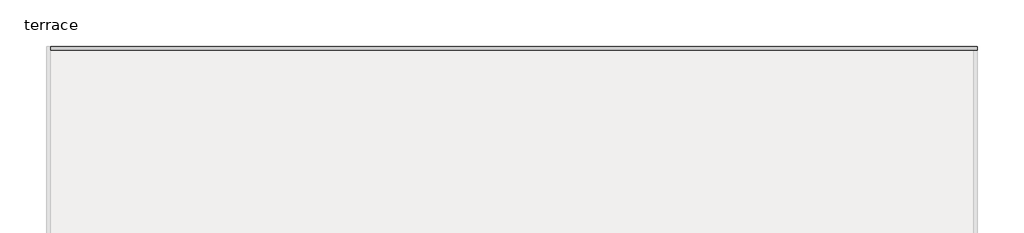
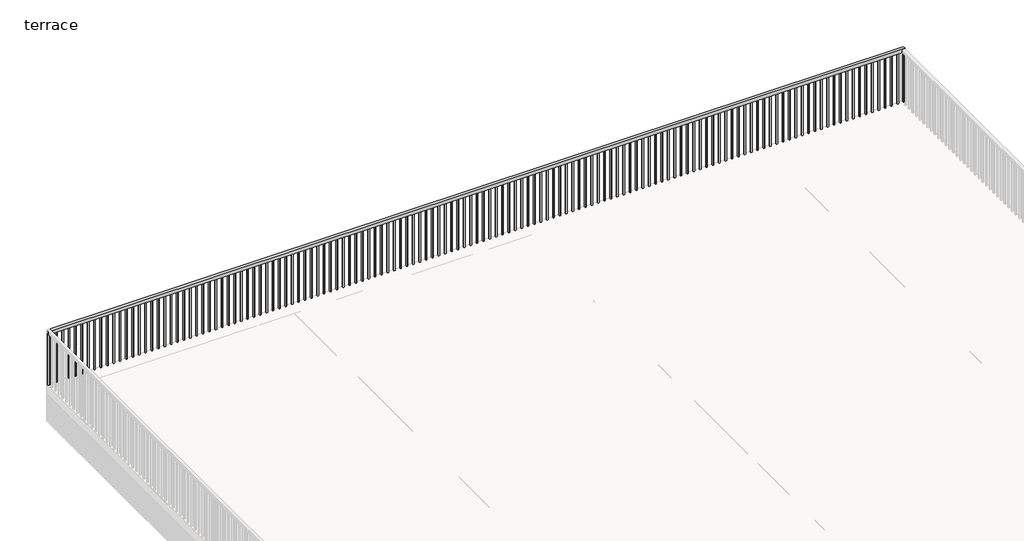
# One storey, part 5 of 6: 1 railing.
"""IFC4 building model written with IfcOpenShell, lengths in millimetres."""

from ifc_helpers import new_model, si_unit, frame, origin, place, context, project, spatial, polyline, outline, extrude, element, save

model = new_model("IFC4")

# Units and contexts
model_context = context("Model", 3, world=origin())
ifc_project = project(units=[si_unit("LENGTHUNIT", "METRE", prefix="MILLI")], contexts=[model_context])

# Site, building, storey
site = spatial("IfcSite", under=ifc_project)
building = spatial("IfcBuilding", under=site)
storey = spatial("IfcBuildingStorey", under=building, Name="terrace", Elevation=7010.4)

# Railing
placement = place(None, origin())
element("IfcRailing", 1, ObjectType="Handrail - Rectangular", at=placement, inside=storey, context=model_context, shape_type="SweptSolid", body=[
    extrude(outline(polyline([(-2647.3594779, 6526.2435985), (-2647.3594779, 6475.4435985), (-16300.5993763, 6475.4435985), (-16300.5993763, 6526.2435985), (-2647.3594779, 6526.2435985)])), frame((0.0, 0.0, 7874.0), z_axis=(0.0, 0.0, 1.0), x_axis=(1.0, 0.0, 0.0)), (0.0, 0.0, 1.0), 50.8),
    extrude(outline(polyline([(-16252.2344779, 6510.3685985), (-16252.2344779, 6491.3185985), (-16271.2844779, 6491.3185985), (-16271.2844779, 6510.3685985), (-16252.2344779, 6510.3685985)])), frame((0.0, 0.0, 7010.4), z_axis=(0.0, 0.0, 1.0), x_axis=(1.0, 0.0, 0.0)), (0.0, 0.0, 1.0), 863.6),
    extrude(outline(polyline([(-16150.6344779, 6510.3685985), (-16150.6344779, 6491.3185985), (-16169.6844779, 6491.3185985), (-16169.6844779, 6510.3685985), (-16150.6344779, 6510.3685985)])), frame((0.0, 0.0, 7010.4), z_axis=(0.0, 0.0, 1.0), x_axis=(1.0, 0.0, 0.0)), (0.0, 0.0, 1.0), 863.6),
    extrude(outline(polyline([(-16049.0344779, 6510.3685985), (-16049.0344779, 6491.3185985), (-16068.0844779, 6491.3185985), (-16068.0844779, 6510.3685985), (-16049.0344779, 6510.3685985)])), frame((0.0, 0.0, 7010.4), z_axis=(0.0, 0.0, 1.0), x_axis=(1.0, 0.0, 0.0)), (0.0, 0.0, 1.0), 863.6),
    extrude(outline(polyline([(-15947.4344779, 6510.3685985), (-15947.4344779, 6491.3185985), (-15966.4844779, 6491.3185985), (-15966.4844779, 6510.3685985), (-15947.4344779, 6510.3685985)])), frame((0.0, 0.0, 7010.4), z_axis=(0.0, 0.0, 1.0), x_axis=(1.0, 0.0, 0.0)), (0.0, 0.0, 1.0), 863.6),
    extrude(outline(polyline([(-15845.8344779, 6510.3685985), (-15845.8344779, 6491.3185985), (-15864.8844779, 6491.3185985), (-15864.8844779, 6510.3685985), (-15845.8344779, 6510.3685985)])), frame((0.0, 0.0, 7010.4), z_axis=(0.0, 0.0, 1.0), x_axis=(1.0, 0.0, 0.0)), (0.0, 0.0, 1.0), 863.6),
    extrude(outline(polyline([(-15744.2344779, 6510.3685985), (-15744.2344779, 6491.3185985), (-15763.2844779, 6491.3185985), (-15763.2844779, 6510.3685985), (-15744.2344779, 6510.3685985)])), frame((0.0, 0.0, 7010.4), z_axis=(0.0, 0.0, 1.0), x_axis=(1.0, 0.0, 0.0)), (0.0, 0.0, 1.0), 863.6),
    extrude(outline(polyline([(-15642.6344779, 6510.3685985), (-15642.6344779, 6491.3185985), (-15661.6844779, 6491.3185985), (-15661.6844779, 6510.3685985), (-15642.6344779, 6510.3685985)])), frame((0.0, 0.0, 7010.4), z_axis=(0.0, 0.0, 1.0), x_axis=(1.0, 0.0, 0.0)), (0.0, 0.0, 1.0), 863.6),
    extrude(outline(polyline([(-15541.0344779, 6510.3685985), (-15541.0344779, 6491.3185985), (-15560.0844779, 6491.3185985), (-15560.0844779, 6510.3685985), (-15541.0344779, 6510.3685985)])), frame((0.0, 0.0, 7010.4), z_axis=(0.0, 0.0, 1.0), x_axis=(1.0, 0.0, 0.0)), (0.0, 0.0, 1.0), 863.6),
    extrude(outline(polyline([(-15439.4344779, 6510.3685985), (-15439.4344779, 6491.3185985), (-15458.4844779, 6491.3185985), (-15458.4844779, 6510.3685985), (-15439.4344779, 6510.3685985)])), frame((0.0, 0.0, 7010.4), z_axis=(0.0, 0.0, 1.0), x_axis=(1.0, 0.0, 0.0)), (0.0, 0.0, 1.0), 863.6),
    extrude(outline(polyline([(-15337.8344779, 6510.3685985), (-15337.8344779, 6491.3185985), (-15356.8844779, 6491.3185985), (-15356.8844779, 6510.3685985), (-15337.8344779, 6510.3685985)])), frame((0.0, 0.0, 7010.4), z_axis=(0.0, 0.0, 1.0), x_axis=(1.0, 0.0, 0.0)), (0.0, 0.0, 1.0), 863.6),
    extrude(outline(polyline([(-15236.2344779, 6510.3685985), (-15236.2344779, 6491.3185985), (-15255.2844779, 6491.3185985), (-15255.2844779, 6510.3685985), (-15236.2344779, 6510.3685985)])), frame((0.0, 0.0, 7010.4), z_axis=(0.0, 0.0, 1.0), x_axis=(1.0, 0.0, 0.0)), (0.0, 0.0, 1.0), 863.6),
    extrude(outline(polyline([(-15134.6344779, 6510.3685985), (-15134.6344779, 6491.3185985), (-15153.6844779, 6491.3185985), (-15153.6844779, 6510.3685985), (-15134.6344779, 6510.3685985)])), frame((0.0, 0.0, 7010.4), z_axis=(0.0, 0.0, 1.0), x_axis=(1.0, 0.0, 0.0)), (0.0, 0.0, 1.0), 863.6),
    extrude(outline(polyline([(-15033.0344779, 6510.3685985), (-15033.0344779, 6491.3185985), (-15052.0844779, 6491.3185985), (-15052.0844779, 6510.3685985), (-15033.0344779, 6510.3685985)])), frame((0.0, 0.0, 7010.4), z_axis=(0.0, 0.0, 1.0), x_axis=(1.0, 0.0, 0.0)), (0.0, 0.0, 1.0), 863.6),
    extrude(outline(polyline([(-14931.4344779, 6510.3685985), (-14931.4344779, 6491.3185985), (-14950.4844779, 6491.3185985), (-14950.4844779, 6510.3685985), (-14931.4344779, 6510.3685985)])), frame((0.0, 0.0, 7010.4), z_axis=(0.0, 0.0, 1.0), x_axis=(1.0, 0.0, 0.0)), (0.0, 0.0, 1.0), 863.6),
    extrude(outline(polyline([(-14829.8344779, 6510.3685985), (-14829.8344779, 6491.3185985), (-14848.8844779, 6491.3185985), (-14848.8844779, 6510.3685985), (-14829.8344779, 6510.3685985)])), frame((0.0, 0.0, 7010.4), z_axis=(0.0, 0.0, 1.0), x_axis=(1.0, 0.0, 0.0)), (0.0, 0.0, 1.0), 863.6),
    extrude(outline(polyline([(-14728.2344779, 6510.3685985), (-14728.2344779, 6491.3185985), (-14747.2844779, 6491.3185985), (-14747.2844779, 6510.3685985), (-14728.2344779, 6510.3685985)])), frame((0.0, 0.0, 7010.4), z_axis=(0.0, 0.0, 1.0), x_axis=(1.0, 0.0, 0.0)), (0.0, 0.0, 1.0), 863.6),
    extrude(outline(polyline([(-14626.6344779, 6510.3685985), (-14626.6344779, 6491.3185985), (-14645.6844779, 6491.3185985), (-14645.6844779, 6510.3685985), (-14626.6344779, 6510.3685985)])), frame((0.0, 0.0, 7010.4), z_axis=(0.0, 0.0, 1.0), x_axis=(1.0, 0.0, 0.0)), (0.0, 0.0, 1.0), 863.6),
    extrude(outline(polyline([(-14525.0344779, 6510.3685985), (-14525.0344779, 6491.3185985), (-14544.0844779, 6491.3185985), (-14544.0844779, 6510.3685985), (-14525.0344779, 6510.3685985)])), frame((0.0, 0.0, 7010.4), z_axis=(0.0, 0.0, 1.0), x_axis=(1.0, 0.0, 0.0)), (0.0, 0.0, 1.0), 863.6),
    extrude(outline(polyline([(-14423.4344779, 6510.3685985), (-14423.4344779, 6491.3185985), (-14442.4844779, 6491.3185985), (-14442.4844779, 6510.3685985), (-14423.4344779, 6510.3685985)])), frame((0.0, 0.0, 7010.4), z_axis=(0.0, 0.0, 1.0), x_axis=(1.0, 0.0, 0.0)), (0.0, 0.0, 1.0), 863.6),
    extrude(outline(polyline([(-14321.8344779, 6510.3685985), (-14321.8344779, 6491.3185985), (-14340.8844779, 6491.3185985), (-14340.8844779, 6510.3685985), (-14321.8344779, 6510.3685985)])), frame((0.0, 0.0, 7010.4), z_axis=(0.0, 0.0, 1.0), x_axis=(1.0, 0.0, 0.0)), (0.0, 0.0, 1.0), 863.6),
    extrude(outline(polyline([(-14220.2344779, 6510.3685985), (-14220.2344779, 6491.3185985), (-14239.2844779, 6491.3185985), (-14239.2844779, 6510.3685985), (-14220.2344779, 6510.3685985)])), frame((0.0, 0.0, 7010.4), z_axis=(0.0, 0.0, 1.0), x_axis=(1.0, 0.0, 0.0)), (0.0, 0.0, 1.0), 863.6),
    extrude(outline(polyline([(-14118.6344779, 6510.3685985), (-14118.6344779, 6491.3185985), (-14137.6844779, 6491.3185985), (-14137.6844779, 6510.3685985), (-14118.6344779, 6510.3685985)])), frame((0.0, 0.0, 7010.4), z_axis=(0.0, 0.0, 1.0), x_axis=(1.0, 0.0, 0.0)), (0.0, 0.0, 1.0), 863.6),
    extrude(outline(polyline([(-14017.0344779, 6510.3685985), (-14017.0344779, 6491.3185985), (-14036.0844779, 6491.3185985), (-14036.0844779, 6510.3685985), (-14017.0344779, 6510.3685985)])), frame((0.0, 0.0, 7010.4), z_axis=(0.0, 0.0, 1.0), x_axis=(1.0, 0.0, 0.0)), (0.0, 0.0, 1.0), 863.6),
    extrude(outline(polyline([(-13915.4344779, 6510.3685985), (-13915.4344779, 6491.3185985), (-13934.4844779, 6491.3185985), (-13934.4844779, 6510.3685985), (-13915.4344779, 6510.3685985)])), frame((0.0, 0.0, 7010.4), z_axis=(0.0, 0.0, 1.0), x_axis=(1.0, 0.0, 0.0)), (0.0, 0.0, 1.0), 863.6),
    extrude(outline(polyline([(-13813.8344779, 6510.3685985), (-13813.8344779, 6491.3185985), (-13832.8844779, 6491.3185985), (-13832.8844779, 6510.3685985), (-13813.8344779, 6510.3685985)])), frame((0.0, 0.0, 7010.4), z_axis=(0.0, 0.0, 1.0), x_axis=(1.0, 0.0, 0.0)), (0.0, 0.0, 1.0), 863.6),
    extrude(outline(polyline([(-13712.2344779, 6510.3685985), (-13712.2344779, 6491.3185985), (-13731.2844779, 6491.3185985), (-13731.2844779, 6510.3685985), (-13712.2344779, 6510.3685985)])), frame((0.0, 0.0, 7010.4), z_axis=(0.0, 0.0, 1.0), x_axis=(1.0, 0.0, 0.0)), (0.0, 0.0, 1.0), 863.6),
    extrude(outline(polyline([(-13610.6344779, 6510.3685985), (-13610.6344779, 6491.3185985), (-13629.6844779, 6491.3185985), (-13629.6844779, 6510.3685985), (-13610.6344779, 6510.3685985)])), frame((0.0, 0.0, 7010.4), z_axis=(0.0, 0.0, 1.0), x_axis=(1.0, 0.0, 0.0)), (0.0, 0.0, 1.0), 863.6),
    extrude(outline(polyline([(-13509.0344779, 6510.3685985), (-13509.0344779, 6491.3185985), (-13528.0844779, 6491.3185985), (-13528.0844779, 6510.3685985), (-13509.0344779, 6510.3685985)])), frame((0.0, 0.0, 7010.4), z_axis=(0.0, 0.0, 1.0), x_axis=(1.0, 0.0, 0.0)), (0.0, 0.0, 1.0), 863.6),
    extrude(outline(polyline([(-13407.4344779, 6510.3685985), (-13407.4344779, 6491.3185985), (-13426.4844779, 6491.3185985), (-13426.4844779, 6510.3685985), (-13407.4344779, 6510.3685985)])), frame((0.0, 0.0, 7010.4), z_axis=(0.0, 0.0, 1.0), x_axis=(1.0, 0.0, 0.0)), (0.0, 0.0, 1.0), 863.6),
    extrude(outline(polyline([(-13305.8344779, 6510.3685985), (-13305.8344779, 6491.3185985), (-13324.8844779, 6491.3185985), (-13324.8844779, 6510.3685985), (-13305.8344779, 6510.3685985)])), frame((0.0, 0.0, 7010.4), z_axis=(0.0, 0.0, 1.0), x_axis=(1.0, 0.0, 0.0)), (0.0, 0.0, 1.0), 863.6),
    extrude(outline(polyline([(-13204.2344779, 6510.3685985), (-13204.2344779, 6491.3185985), (-13223.2844779, 6491.3185985), (-13223.2844779, 6510.3685985), (-13204.2344779, 6510.3685985)])), frame((0.0, 0.0, 7010.4), z_axis=(0.0, 0.0, 1.0), x_axis=(1.0, 0.0, 0.0)), (0.0, 0.0, 1.0), 863.6),
    extrude(outline(polyline([(-13102.6344779, 6510.3685985), (-13102.6344779, 6491.3185985), (-13121.6844779, 6491.3185985), (-13121.6844779, 6510.3685985), (-13102.6344779, 6510.3685985)])), frame((0.0, 0.0, 7010.4), z_axis=(0.0, 0.0, 1.0), x_axis=(1.0, 0.0, 0.0)), (0.0, 0.0, 1.0), 863.6),
    extrude(outline(polyline([(-13001.0344779, 6510.3685985), (-13001.0344779, 6491.3185985), (-13020.0844779, 6491.3185985), (-13020.0844779, 6510.3685985), (-13001.0344779, 6510.3685985)])), frame((0.0, 0.0, 7010.4), z_axis=(0.0, 0.0, 1.0), x_axis=(1.0, 0.0, 0.0)), (0.0, 0.0, 1.0), 863.6),
    extrude(outline(polyline([(-12899.4344779, 6510.3685985), (-12899.4344779, 6491.3185985), (-12918.4844779, 6491.3185985), (-12918.4844779, 6510.3685985), (-12899.4344779, 6510.3685985)])), frame((0.0, 0.0, 7010.4), z_axis=(0.0, 0.0, 1.0), x_axis=(1.0, 0.0, 0.0)), (0.0, 0.0, 1.0), 863.6),
    extrude(outline(polyline([(-12797.8344779, 6510.3685985), (-12797.8344779, 6491.3185985), (-12816.8844779, 6491.3185985), (-12816.8844779, 6510.3685985), (-12797.8344779, 6510.3685985)])), frame((0.0, 0.0, 7010.4), z_axis=(0.0, 0.0, 1.0), x_axis=(1.0, 0.0, 0.0)), (0.0, 0.0, 1.0), 863.6),
    extrude(outline(polyline([(-12696.2344779, 6510.3685985), (-12696.2344779, 6491.3185985), (-12715.2844779, 6491.3185985), (-12715.2844779, 6510.3685985), (-12696.2344779, 6510.3685985)])), frame((0.0, 0.0, 7010.4), z_axis=(0.0, 0.0, 1.0), x_axis=(1.0, 0.0, 0.0)), (0.0, 0.0, 1.0), 863.6),
    extrude(outline(polyline([(-12594.6344779, 6510.3685985), (-12594.6344779, 6491.3185985), (-12613.6844779, 6491.3185985), (-12613.6844779, 6510.3685985), (-12594.6344779, 6510.3685985)])), frame((0.0, 0.0, 7010.4), z_axis=(0.0, 0.0, 1.0), x_axis=(1.0, 0.0, 0.0)), (0.0, 0.0, 1.0), 863.6),
    extrude(outline(polyline([(-12493.0344779, 6510.3685985), (-12493.0344779, 6491.3185985), (-12512.0844779, 6491.3185985), (-12512.0844779, 6510.3685985), (-12493.0344779, 6510.3685985)])), frame((0.0, 0.0, 7010.4), z_axis=(0.0, 0.0, 1.0), x_axis=(1.0, 0.0, 0.0)), (0.0, 0.0, 1.0), 863.6),
    extrude(outline(polyline([(-12391.4344779, 6510.3685985), (-12391.4344779, 6491.3185985), (-12410.4844779, 6491.3185985), (-12410.4844779, 6510.3685985), (-12391.4344779, 6510.3685985)])), frame((0.0, 0.0, 7010.4), z_axis=(0.0, 0.0, 1.0), x_axis=(1.0, 0.0, 0.0)), (0.0, 0.0, 1.0), 863.6),
    extrude(outline(polyline([(-12289.8344779, 6510.3685985), (-12289.8344779, 6491.3185985), (-12308.8844779, 6491.3185985), (-12308.8844779, 6510.3685985), (-12289.8344779, 6510.3685985)])), frame((0.0, 0.0, 7010.4), z_axis=(0.0, 0.0, 1.0), x_axis=(1.0, 0.0, 0.0)), (0.0, 0.0, 1.0), 863.6),
    extrude(outline(polyline([(-12188.2344779, 6510.3685985), (-12188.2344779, 6491.3185985), (-12207.2844779, 6491.3185985), (-12207.2844779, 6510.3685985), (-12188.2344779, 6510.3685985)])), frame((0.0, 0.0, 7010.4), z_axis=(0.0, 0.0, 1.0), x_axis=(1.0, 0.0, 0.0)), (0.0, 0.0, 1.0), 863.6),
    extrude(outline(polyline([(-12086.6344779, 6510.3685985), (-12086.6344779, 6491.3185985), (-12105.6844779, 6491.3185985), (-12105.6844779, 6510.3685985), (-12086.6344779, 6510.3685985)])), frame((0.0, 0.0, 7010.4), z_axis=(0.0, 0.0, 1.0), x_axis=(1.0, 0.0, 0.0)), (0.0, 0.0, 1.0), 863.6),
    extrude(outline(polyline([(-11985.0344779, 6510.3685985), (-11985.0344779, 6491.3185985), (-12004.0844779, 6491.3185985), (-12004.0844779, 6510.3685985), (-11985.0344779, 6510.3685985)])), frame((0.0, 0.0, 7010.4), z_axis=(0.0, 0.0, 1.0), x_axis=(1.0, 0.0, 0.0)), (0.0, 0.0, 1.0), 863.6),
    extrude(outline(polyline([(-11883.4344779, 6510.3685985), (-11883.4344779, 6491.3185985), (-11902.4844779, 6491.3185985), (-11902.4844779, 6510.3685985), (-11883.4344779, 6510.3685985)])), frame((0.0, 0.0, 7010.4), z_axis=(0.0, 0.0, 1.0), x_axis=(1.0, 0.0, 0.0)), (0.0, 0.0, 1.0), 863.6),
    extrude(outline(polyline([(-11781.8344779, 6510.3685985), (-11781.8344779, 6491.3185985), (-11800.8844779, 6491.3185985), (-11800.8844779, 6510.3685985), (-11781.8344779, 6510.3685985)])), frame((0.0, 0.0, 7010.4), z_axis=(0.0, 0.0, 1.0), x_axis=(1.0, 0.0, 0.0)), (0.0, 0.0, 1.0), 863.6),
    extrude(outline(polyline([(-11680.2344779, 6510.3685985), (-11680.2344779, 6491.3185985), (-11699.2844779, 6491.3185985), (-11699.2844779, 6510.3685985), (-11680.2344779, 6510.3685985)])), frame((0.0, 0.0, 7010.4), z_axis=(0.0, 0.0, 1.0), x_axis=(1.0, 0.0, 0.0)), (0.0, 0.0, 1.0), 863.6),
    extrude(outline(polyline([(-11578.6344779, 6510.3685985), (-11578.6344779, 6491.3185985), (-11597.6844779, 6491.3185985), (-11597.6844779, 6510.3685985), (-11578.6344779, 6510.3685985)])), frame((0.0, 0.0, 7010.4), z_axis=(0.0, 0.0, 1.0), x_axis=(1.0, 0.0, 0.0)), (0.0, 0.0, 1.0), 863.6),
    extrude(outline(polyline([(-11477.0344779, 6510.3685985), (-11477.0344779, 6491.3185985), (-11496.0844779, 6491.3185985), (-11496.0844779, 6510.3685985), (-11477.0344779, 6510.3685985)])), frame((0.0, 0.0, 7010.4), z_axis=(0.0, 0.0, 1.0), x_axis=(1.0, 0.0, 0.0)), (0.0, 0.0, 1.0), 863.6),
    extrude(outline(polyline([(-11375.4344779, 6510.3685985), (-11375.4344779, 6491.3185985), (-11394.4844779, 6491.3185985), (-11394.4844779, 6510.3685985), (-11375.4344779, 6510.3685985)])), frame((0.0, 0.0, 7010.4), z_axis=(0.0, 0.0, 1.0), x_axis=(1.0, 0.0, 0.0)), (0.0, 0.0, 1.0), 863.6),
    extrude(outline(polyline([(-11273.8344779, 6510.3685985), (-11273.8344779, 6491.3185985), (-11292.8844779, 6491.3185985), (-11292.8844779, 6510.3685985), (-11273.8344779, 6510.3685985)])), frame((0.0, 0.0, 7010.4), z_axis=(0.0, 0.0, 1.0), x_axis=(1.0, 0.0, 0.0)), (0.0, 0.0, 1.0), 863.6),
    extrude(outline(polyline([(-11172.2344779, 6510.3685985), (-11172.2344779, 6491.3185985), (-11191.2844779, 6491.3185985), (-11191.2844779, 6510.3685985), (-11172.2344779, 6510.3685985)])), frame((0.0, 0.0, 7010.4), z_axis=(0.0, 0.0, 1.0), x_axis=(1.0, 0.0, 0.0)), (0.0, 0.0, 1.0), 863.6),
    extrude(outline(polyline([(-11070.6344779, 6510.3685985), (-11070.6344779, 6491.3185985), (-11089.6844779, 6491.3185985), (-11089.6844779, 6510.3685985), (-11070.6344779, 6510.3685985)])), frame((0.0, 0.0, 7010.4), z_axis=(0.0, 0.0, 1.0), x_axis=(1.0, 0.0, 0.0)), (0.0, 0.0, 1.0), 863.6),
    extrude(outline(polyline([(-10969.0344779, 6510.3685985), (-10969.0344779, 6491.3185985), (-10988.0844779, 6491.3185985), (-10988.0844779, 6510.3685985), (-10969.0344779, 6510.3685985)])), frame((0.0, 0.0, 7010.4), z_axis=(0.0, 0.0, 1.0), x_axis=(1.0, 0.0, 0.0)), (0.0, 0.0, 1.0), 863.6),
    extrude(outline(polyline([(-10867.4344779, 6510.3685985), (-10867.4344779, 6491.3185985), (-10886.4844779, 6491.3185985), (-10886.4844779, 6510.3685985), (-10867.4344779, 6510.3685985)])), frame((0.0, 0.0, 7010.4), z_axis=(0.0, 0.0, 1.0), x_axis=(1.0, 0.0, 0.0)), (0.0, 0.0, 1.0), 863.6),
    extrude(outline(polyline([(-10765.8344779, 6510.3685985), (-10765.8344779, 6491.3185985), (-10784.8844779, 6491.3185985), (-10784.8844779, 6510.3685985), (-10765.8344779, 6510.3685985)])), frame((0.0, 0.0, 7010.4), z_axis=(0.0, 0.0, 1.0), x_axis=(1.0, 0.0, 0.0)), (0.0, 0.0, 1.0), 863.6),
    extrude(outline(polyline([(-10664.2344779, 6510.3685985), (-10664.2344779, 6491.3185985), (-10683.2844779, 6491.3185985), (-10683.2844779, 6510.3685985), (-10664.2344779, 6510.3685985)])), frame((0.0, 0.0, 7010.4), z_axis=(0.0, 0.0, 1.0), x_axis=(1.0, 0.0, 0.0)), (0.0, 0.0, 1.0), 863.6),
    extrude(outline(polyline([(-10562.6344779, 6510.3685985), (-10562.6344779, 6491.3185985), (-10581.6844779, 6491.3185985), (-10581.6844779, 6510.3685985), (-10562.6344779, 6510.3685985)])), frame((0.0, 0.0, 7010.4), z_axis=(0.0, 0.0, 1.0), x_axis=(1.0, 0.0, 0.0)), (0.0, 0.0, 1.0), 863.6),
    extrude(outline(polyline([(-10461.0344779, 6510.3685985), (-10461.0344779, 6491.3185985), (-10480.0844779, 6491.3185985), (-10480.0844779, 6510.3685985), (-10461.0344779, 6510.3685985)])), frame((0.0, 0.0, 7010.4), z_axis=(0.0, 0.0, 1.0), x_axis=(1.0, 0.0, 0.0)), (0.0, 0.0, 1.0), 863.6),
    extrude(outline(polyline([(-10359.4344779, 6510.3685985), (-10359.4344779, 6491.3185985), (-10378.4844779, 6491.3185985), (-10378.4844779, 6510.3685985), (-10359.4344779, 6510.3685985)])), frame((0.0, 0.0, 7010.4), z_axis=(0.0, 0.0, 1.0), x_axis=(1.0, 0.0, 0.0)), (0.0, 0.0, 1.0), 863.6),
    extrude(outline(polyline([(-10257.8344779, 6510.3685985), (-10257.8344779, 6491.3185985), (-10276.8844779, 6491.3185985), (-10276.8844779, 6510.3685985), (-10257.8344779, 6510.3685985)])), frame((0.0, 0.0, 7010.4), z_axis=(0.0, 0.0, 1.0), x_axis=(1.0, 0.0, 0.0)), (0.0, 0.0, 1.0), 863.6),
    extrude(outline(polyline([(-10156.2344779, 6510.3685985), (-10156.2344779, 6491.3185985), (-10175.2844779, 6491.3185985), (-10175.2844779, 6510.3685985), (-10156.2344779, 6510.3685985)])), frame((0.0, 0.0, 7010.4), z_axis=(0.0, 0.0, 1.0), x_axis=(1.0, 0.0, 0.0)), (0.0, 0.0, 1.0), 863.6),
    extrude(outline(polyline([(-10054.6344779, 6510.3685985), (-10054.6344779, 6491.3185985), (-10073.6844779, 6491.3185985), (-10073.6844779, 6510.3685985), (-10054.6344779, 6510.3685985)])), frame((0.0, 0.0, 7010.4), z_axis=(0.0, 0.0, 1.0), x_axis=(1.0, 0.0, 0.0)), (0.0, 0.0, 1.0), 863.6),
    extrude(outline(polyline([(-9953.0344779, 6510.3685985), (-9953.0344779, 6491.3185985), (-9972.0844779, 6491.3185985), (-9972.0844779, 6510.3685985), (-9953.0344779, 6510.3685985)])), frame((0.0, 0.0, 7010.4), z_axis=(0.0, 0.0, 1.0), x_axis=(1.0, 0.0, 0.0)), (0.0, 0.0, 1.0), 863.6),
    extrude(outline(polyline([(-9851.4344779, 6510.3685985), (-9851.4344779, 6491.3185985), (-9870.4844779, 6491.3185985), (-9870.4844779, 6510.3685985), (-9851.4344779, 6510.3685985)])), frame((0.0, 0.0, 7010.4), z_axis=(0.0, 0.0, 1.0), x_axis=(1.0, 0.0, 0.0)), (0.0, 0.0, 1.0), 863.6),
    extrude(outline(polyline([(-9749.8344779, 6510.3685985), (-9749.8344779, 6491.3185985), (-9768.8844779, 6491.3185985), (-9768.8844779, 6510.3685985), (-9749.8344779, 6510.3685985)])), frame((0.0, 0.0, 7010.4), z_axis=(0.0, 0.0, 1.0), x_axis=(1.0, 0.0, 0.0)), (0.0, 0.0, 1.0), 863.6),
    extrude(outline(polyline([(-9648.2344779, 6510.3685985), (-9648.2344779, 6491.3185985), (-9667.2844779, 6491.3185985), (-9667.2844779, 6510.3685985), (-9648.2344779, 6510.3685985)])), frame((0.0, 0.0, 7010.4), z_axis=(0.0, 0.0, 1.0), x_axis=(1.0, 0.0, 0.0)), (0.0, 0.0, 1.0), 863.6),
    extrude(outline(polyline([(-9546.6344779, 6510.3685985), (-9546.6344779, 6491.3185985), (-9565.6844779, 6491.3185985), (-9565.6844779, 6510.3685985), (-9546.6344779, 6510.3685985)])), frame((0.0, 0.0, 7010.4), z_axis=(0.0, 0.0, 1.0), x_axis=(1.0, 0.0, 0.0)), (0.0, 0.0, 1.0), 863.6),
    extrude(outline(polyline([(-9445.0344779, 6510.3685985), (-9445.0344779, 6491.3185985), (-9464.0844779, 6491.3185985), (-9464.0844779, 6510.3685985), (-9445.0344779, 6510.3685985)])), frame((0.0, 0.0, 7010.4), z_axis=(0.0, 0.0, 1.0), x_axis=(1.0, 0.0, 0.0)), (0.0, 0.0, 1.0), 863.6),
    extrude(outline(polyline([(-9343.4344779, 6510.3685985), (-9343.4344779, 6491.3185985), (-9362.4844779, 6491.3185985), (-9362.4844779, 6510.3685985), (-9343.4344779, 6510.3685985)])), frame((0.0, 0.0, 7010.4), z_axis=(0.0, 0.0, 1.0), x_axis=(1.0, 0.0, 0.0)), (0.0, 0.0, 1.0), 863.6),
    extrude(outline(polyline([(-9241.8344779, 6510.3685985), (-9241.8344779, 6491.3185985), (-9260.8844779, 6491.3185985), (-9260.8844779, 6510.3685985), (-9241.8344779, 6510.3685985)])), frame((0.0, 0.0, 7010.4), z_axis=(0.0, 0.0, 1.0), x_axis=(1.0, 0.0, 0.0)), (0.0, 0.0, 1.0), 863.6),
    extrude(outline(polyline([(-9140.2344779, 6510.3685985), (-9140.2344779, 6491.3185985), (-9159.2844779, 6491.3185985), (-9159.2844779, 6510.3685985), (-9140.2344779, 6510.3685985)])), frame((0.0, 0.0, 7010.4), z_axis=(0.0, 0.0, 1.0), x_axis=(1.0, 0.0, 0.0)), (0.0, 0.0, 1.0), 863.6),
    extrude(outline(polyline([(-9038.6344779, 6510.3685985), (-9038.6344779, 6491.3185985), (-9057.6844779, 6491.3185985), (-9057.6844779, 6510.3685985), (-9038.6344779, 6510.3685985)])), frame((0.0, 0.0, 7010.4), z_axis=(0.0, 0.0, 1.0), x_axis=(1.0, 0.0, 0.0)), (0.0, 0.0, 1.0), 863.6),
    extrude(outline(polyline([(-8937.0344779, 6510.3685985), (-8937.0344779, 6491.3185985), (-8956.0844779, 6491.3185985), (-8956.0844779, 6510.3685985), (-8937.0344779, 6510.3685985)])), frame((0.0, 0.0, 7010.4), z_axis=(0.0, 0.0, 1.0), x_axis=(1.0, 0.0, 0.0)), (0.0, 0.0, 1.0), 863.6),
    extrude(outline(polyline([(-8835.4344779, 6510.3685985), (-8835.4344779, 6491.3185985), (-8854.4844779, 6491.3185985), (-8854.4844779, 6510.3685985), (-8835.4344779, 6510.3685985)])), frame((0.0, 0.0, 7010.4), z_axis=(0.0, 0.0, 1.0), x_axis=(1.0, 0.0, 0.0)), (0.0, 0.0, 1.0), 863.6),
    extrude(outline(polyline([(-8733.8344779, 6510.3685985), (-8733.8344779, 6491.3185985), (-8752.8844779, 6491.3185985), (-8752.8844779, 6510.3685985), (-8733.8344779, 6510.3685985)])), frame((0.0, 0.0, 7010.4), z_axis=(0.0, 0.0, 1.0), x_axis=(1.0, 0.0, 0.0)), (0.0, 0.0, 1.0), 863.6),
    extrude(outline(polyline([(-8632.2344779, 6510.3685985), (-8632.2344779, 6491.3185985), (-8651.2844779, 6491.3185985), (-8651.2844779, 6510.3685985), (-8632.2344779, 6510.3685985)])), frame((0.0, 0.0, 7010.4), z_axis=(0.0, 0.0, 1.0), x_axis=(1.0, 0.0, 0.0)), (0.0, 0.0, 1.0), 863.6),
    extrude(outline(polyline([(-8530.6344779, 6510.3685985), (-8530.6344779, 6491.3185985), (-8549.6844779, 6491.3185985), (-8549.6844779, 6510.3685985), (-8530.6344779, 6510.3685985)])), frame((0.0, 0.0, 7010.4), z_axis=(0.0, 0.0, 1.0), x_axis=(1.0, 0.0, 0.0)), (0.0, 0.0, 1.0), 863.6),
    extrude(outline(polyline([(-8429.0344779, 6510.3685985), (-8429.0344779, 6491.3185985), (-8448.0844779, 6491.3185985), (-8448.0844779, 6510.3685985), (-8429.0344779, 6510.3685985)])), frame((0.0, 0.0, 7010.4), z_axis=(0.0, 0.0, 1.0), x_axis=(1.0, 0.0, 0.0)), (0.0, 0.0, 1.0), 863.6),
    extrude(outline(polyline([(-8327.4344779, 6510.3685985), (-8327.4344779, 6491.3185985), (-8346.4844779, 6491.3185985), (-8346.4844779, 6510.3685985), (-8327.4344779, 6510.3685985)])), frame((0.0, 0.0, 7010.4), z_axis=(0.0, 0.0, 1.0), x_axis=(1.0, 0.0, 0.0)), (0.0, 0.0, 1.0), 863.6),
    extrude(outline(polyline([(-8225.8344779, 6510.3685985), (-8225.8344779, 6491.3185985), (-8244.8844779, 6491.3185985), (-8244.8844779, 6510.3685985), (-8225.8344779, 6510.3685985)])), frame((0.0, 0.0, 7010.4), z_axis=(0.0, 0.0, 1.0), x_axis=(1.0, 0.0, 0.0)), (0.0, 0.0, 1.0), 863.6),
    extrude(outline(polyline([(-8124.2344779, 6510.3685985), (-8124.2344779, 6491.3185985), (-8143.2844779, 6491.3185985), (-8143.2844779, 6510.3685985), (-8124.2344779, 6510.3685985)])), frame((0.0, 0.0, 7010.4), z_axis=(0.0, 0.0, 1.0), x_axis=(1.0, 0.0, 0.0)), (0.0, 0.0, 1.0), 863.6),
    extrude(outline(polyline([(-8022.6344779, 6510.3685985), (-8022.6344779, 6491.3185985), (-8041.6844779, 6491.3185985), (-8041.6844779, 6510.3685985), (-8022.6344779, 6510.3685985)])), frame((0.0, 0.0, 7010.4), z_axis=(0.0, 0.0, 1.0), x_axis=(1.0, 0.0, 0.0)), (0.0, 0.0, 1.0), 863.6),
    extrude(outline(polyline([(-7921.0344779, 6510.3685985), (-7921.0344779, 6491.3185985), (-7940.0844779, 6491.3185985), (-7940.0844779, 6510.3685985), (-7921.0344779, 6510.3685985)])), frame((0.0, 0.0, 7010.4), z_axis=(0.0, 0.0, 1.0), x_axis=(1.0, 0.0, 0.0)), (0.0, 0.0, 1.0), 863.6),
    extrude(outline(polyline([(-7819.4344779, 6510.3685985), (-7819.4344779, 6491.3185985), (-7838.4844779, 6491.3185985), (-7838.4844779, 6510.3685985), (-7819.4344779, 6510.3685985)])), frame((0.0, 0.0, 7010.4), z_axis=(0.0, 0.0, 1.0), x_axis=(1.0, 0.0, 0.0)), (0.0, 0.0, 1.0), 863.6),
    extrude(outline(polyline([(-7717.8344779, 6510.3685985), (-7717.8344779, 6491.3185985), (-7736.8844779, 6491.3185985), (-7736.8844779, 6510.3685985), (-7717.8344779, 6510.3685985)])), frame((0.0, 0.0, 7010.4), z_axis=(0.0, 0.0, 1.0), x_axis=(1.0, 0.0, 0.0)), (0.0, 0.0, 1.0), 863.6),
    extrude(outline(polyline([(-7616.2344779, 6510.3685985), (-7616.2344779, 6491.3185985), (-7635.2844779, 6491.3185985), (-7635.2844779, 6510.3685985), (-7616.2344779, 6510.3685985)])), frame((0.0, 0.0, 7010.4), z_axis=(0.0, 0.0, 1.0), x_axis=(1.0, 0.0, 0.0)), (0.0, 0.0, 1.0), 863.6),
    extrude(outline(polyline([(-7514.6344779, 6510.3685985), (-7514.6344779, 6491.3185985), (-7533.6844779, 6491.3185985), (-7533.6844779, 6510.3685985), (-7514.6344779, 6510.3685985)])), frame((0.0, 0.0, 7010.4), z_axis=(0.0, 0.0, 1.0), x_axis=(1.0, 0.0, 0.0)), (0.0, 0.0, 1.0), 863.6),
    extrude(outline(polyline([(-7413.0344779, 6510.3685985), (-7413.0344779, 6491.3185985), (-7432.0844779, 6491.3185985), (-7432.0844779, 6510.3685985), (-7413.0344779, 6510.3685985)])), frame((0.0, 0.0, 7010.4), z_axis=(0.0, 0.0, 1.0), x_axis=(1.0, 0.0, 0.0)), (0.0, 0.0, 1.0), 863.6),
    extrude(outline(polyline([(-7311.4344779, 6510.3685985), (-7311.4344779, 6491.3185985), (-7330.4844779, 6491.3185985), (-7330.4844779, 6510.3685985), (-7311.4344779, 6510.3685985)])), frame((0.0, 0.0, 7010.4), z_axis=(0.0, 0.0, 1.0), x_axis=(1.0, 0.0, 0.0)), (0.0, 0.0, 1.0), 863.6),
    extrude(outline(polyline([(-7209.8344779, 6510.3685985), (-7209.8344779, 6491.3185985), (-7228.8844779, 6491.3185985), (-7228.8844779, 6510.3685985), (-7209.8344779, 6510.3685985)])), frame((0.0, 0.0, 7010.4), z_axis=(0.0, 0.0, 1.0), x_axis=(1.0, 0.0, 0.0)), (0.0, 0.0, 1.0), 863.6),
    extrude(outline(polyline([(-7108.2344779, 6510.3685985), (-7108.2344779, 6491.3185985), (-7127.2844779, 6491.3185985), (-7127.2844779, 6510.3685985), (-7108.2344779, 6510.3685985)])), frame((0.0, 0.0, 7010.4), z_axis=(0.0, 0.0, 1.0), x_axis=(1.0, 0.0, 0.0)), (0.0, 0.0, 1.0), 863.6),
    extrude(outline(polyline([(-7006.6344779, 6510.3685985), (-7006.6344779, 6491.3185985), (-7025.6844779, 6491.3185985), (-7025.6844779, 6510.3685985), (-7006.6344779, 6510.3685985)])), frame((0.0, 0.0, 7010.4), z_axis=(0.0, 0.0, 1.0), x_axis=(1.0, 0.0, 0.0)), (0.0, 0.0, 1.0), 863.6),
    extrude(outline(polyline([(-6905.0344779, 6510.3685985), (-6905.0344779, 6491.3185985), (-6924.0844779, 6491.3185985), (-6924.0844779, 6510.3685985), (-6905.0344779, 6510.3685985)])), frame((0.0, 0.0, 7010.4), z_axis=(0.0, 0.0, 1.0), x_axis=(1.0, 0.0, 0.0)), (0.0, 0.0, 1.0), 863.6),
    extrude(outline(polyline([(-6803.4344779, 6510.3685985), (-6803.4344779, 6491.3185985), (-6822.4844779, 6491.3185985), (-6822.4844779, 6510.3685985), (-6803.4344779, 6510.3685985)])), frame((0.0, 0.0, 7010.4), z_axis=(0.0, 0.0, 1.0), x_axis=(1.0, 0.0, 0.0)), (0.0, 0.0, 1.0), 863.6),
    extrude(outline(polyline([(-6701.8344779, 6510.3685985), (-6701.8344779, 6491.3185985), (-6720.8844779, 6491.3185985), (-6720.8844779, 6510.3685985), (-6701.8344779, 6510.3685985)])), frame((0.0, 0.0, 7010.4), z_axis=(0.0, 0.0, 1.0), x_axis=(1.0, 0.0, 0.0)), (0.0, 0.0, 1.0), 863.6),
    extrude(outline(polyline([(-6600.2344779, 6510.3685985), (-6600.2344779, 6491.3185985), (-6619.2844779, 6491.3185985), (-6619.2844779, 6510.3685985), (-6600.2344779, 6510.3685985)])), frame((0.0, 0.0, 7010.4), z_axis=(0.0, 0.0, 1.0), x_axis=(1.0, 0.0, 0.0)), (0.0, 0.0, 1.0), 863.6),
    extrude(outline(polyline([(-6498.6344779, 6510.3685985), (-6498.6344779, 6491.3185985), (-6517.6844779, 6491.3185985), (-6517.6844779, 6510.3685985), (-6498.6344779, 6510.3685985)])), frame((0.0, 0.0, 7010.4), z_axis=(0.0, 0.0, 1.0), x_axis=(1.0, 0.0, 0.0)), (0.0, 0.0, 1.0), 863.6),
    extrude(outline(polyline([(-6397.0344779, 6510.3685985), (-6397.0344779, 6491.3185985), (-6416.0844779, 6491.3185985), (-6416.0844779, 6510.3685985), (-6397.0344779, 6510.3685985)])), frame((0.0, 0.0, 7010.4), z_axis=(0.0, 0.0, 1.0), x_axis=(1.0, 0.0, 0.0)), (0.0, 0.0, 1.0), 863.6),
    extrude(outline(polyline([(-6295.4344779, 6510.3685985), (-6295.4344779, 6491.3185985), (-6314.4844779, 6491.3185985), (-6314.4844779, 6510.3685985), (-6295.4344779, 6510.3685985)])), frame((0.0, 0.0, 7010.4), z_axis=(0.0, 0.0, 1.0), x_axis=(1.0, 0.0, 0.0)), (0.0, 0.0, 1.0), 863.6),
    extrude(outline(polyline([(-6193.8344779, 6510.3685985), (-6193.8344779, 6491.3185985), (-6212.8844779, 6491.3185985), (-6212.8844779, 6510.3685985), (-6193.8344779, 6510.3685985)])), frame((0.0, 0.0, 7010.4), z_axis=(0.0, 0.0, 1.0), x_axis=(1.0, 0.0, 0.0)), (0.0, 0.0, 1.0), 863.6),
    extrude(outline(polyline([(-6092.2344779, 6510.3685985), (-6092.2344779, 6491.3185985), (-6111.2844779, 6491.3185985), (-6111.2844779, 6510.3685985), (-6092.2344779, 6510.3685985)])), frame((0.0, 0.0, 7010.4), z_axis=(0.0, 0.0, 1.0), x_axis=(1.0, 0.0, 0.0)), (0.0, 0.0, 1.0), 863.6),
    extrude(outline(polyline([(-5990.6344779, 6510.3685985), (-5990.6344779, 6491.3185985), (-6009.6844779, 6491.3185985), (-6009.6844779, 6510.3685985), (-5990.6344779, 6510.3685985)])), frame((0.0, 0.0, 7010.4), z_axis=(0.0, 0.0, 1.0), x_axis=(1.0, 0.0, 0.0)), (0.0, 0.0, 1.0), 863.6),
    extrude(outline(polyline([(-5889.0344779, 6510.3685985), (-5889.0344779, 6491.3185985), (-5908.0844779, 6491.3185985), (-5908.0844779, 6510.3685985), (-5889.0344779, 6510.3685985)])), frame((0.0, 0.0, 7010.4), z_axis=(0.0, 0.0, 1.0), x_axis=(1.0, 0.0, 0.0)), (0.0, 0.0, 1.0), 863.6),
    extrude(outline(polyline([(-5787.4344779, 6510.3685985), (-5787.4344779, 6491.3185985), (-5806.4844779, 6491.3185985), (-5806.4844779, 6510.3685985), (-5787.4344779, 6510.3685985)])), frame((0.0, 0.0, 7010.4), z_axis=(0.0, 0.0, 1.0), x_axis=(1.0, 0.0, 0.0)), (0.0, 0.0, 1.0), 863.6),
    extrude(outline(polyline([(-5685.8344779, 6510.3685985), (-5685.8344779, 6491.3185985), (-5704.8844779, 6491.3185985), (-5704.8844779, 6510.3685985), (-5685.8344779, 6510.3685985)])), frame((0.0, 0.0, 7010.4), z_axis=(0.0, 0.0, 1.0), x_axis=(1.0, 0.0, 0.0)), (0.0, 0.0, 1.0), 863.6),
    extrude(outline(polyline([(-5584.2344779, 6510.3685985), (-5584.2344779, 6491.3185985), (-5603.2844779, 6491.3185985), (-5603.2844779, 6510.3685985), (-5584.2344779, 6510.3685985)])), frame((0.0, 0.0, 7010.4), z_axis=(0.0, 0.0, 1.0), x_axis=(1.0, 0.0, 0.0)), (0.0, 0.0, 1.0), 863.6),
    extrude(outline(polyline([(-5482.6344779, 6510.3685985), (-5482.6344779, 6491.3185985), (-5501.6844779, 6491.3185985), (-5501.6844779, 6510.3685985), (-5482.6344779, 6510.3685985)])), frame((0.0, 0.0, 7010.4), z_axis=(0.0, 0.0, 1.0), x_axis=(1.0, 0.0, 0.0)), (0.0, 0.0, 1.0), 863.6),
    extrude(outline(polyline([(-5381.0344779, 6510.3685985), (-5381.0344779, 6491.3185985), (-5400.0844779, 6491.3185985), (-5400.0844779, 6510.3685985), (-5381.0344779, 6510.3685985)])), frame((0.0, 0.0, 7010.4), z_axis=(0.0, 0.0, 1.0), x_axis=(1.0, 0.0, 0.0)), (0.0, 0.0, 1.0), 863.6),
    extrude(outline(polyline([(-5279.4344779, 6510.3685985), (-5279.4344779, 6491.3185985), (-5298.4844779, 6491.3185985), (-5298.4844779, 6510.3685985), (-5279.4344779, 6510.3685985)])), frame((0.0, 0.0, 7010.4), z_axis=(0.0, 0.0, 1.0), x_axis=(1.0, 0.0, 0.0)), (0.0, 0.0, 1.0), 863.6),
    extrude(outline(polyline([(-5177.8344779, 6510.3685985), (-5177.8344779, 6491.3185985), (-5196.8844779, 6491.3185985), (-5196.8844779, 6510.3685985), (-5177.8344779, 6510.3685985)])), frame((0.0, 0.0, 7010.4), z_axis=(0.0, 0.0, 1.0), x_axis=(1.0, 0.0, 0.0)), (0.0, 0.0, 1.0), 863.6),
    extrude(outline(polyline([(-5076.2344779, 6510.3685985), (-5076.2344779, 6491.3185985), (-5095.2844779, 6491.3185985), (-5095.2844779, 6510.3685985), (-5076.2344779, 6510.3685985)])), frame((0.0, 0.0, 7010.4), z_axis=(0.0, 0.0, 1.0), x_axis=(1.0, 0.0, 0.0)), (0.0, 0.0, 1.0), 863.6),
    extrude(outline(polyline([(-4974.6344779, 6510.3685985), (-4974.6344779, 6491.3185985), (-4993.6844779, 6491.3185985), (-4993.6844779, 6510.3685985), (-4974.6344779, 6510.3685985)])), frame((0.0, 0.0, 7010.4), z_axis=(0.0, 0.0, 1.0), x_axis=(1.0, 0.0, 0.0)), (0.0, 0.0, 1.0), 863.6),
    extrude(outline(polyline([(-4873.0344779, 6510.3685985), (-4873.0344779, 6491.3185985), (-4892.0844779, 6491.3185985), (-4892.0844779, 6510.3685985), (-4873.0344779, 6510.3685985)])), frame((0.0, 0.0, 7010.4), z_axis=(0.0, 0.0, 1.0), x_axis=(1.0, 0.0, 0.0)), (0.0, 0.0, 1.0), 863.6),
    extrude(outline(polyline([(-4771.4344779, 6510.3685985), (-4771.4344779, 6491.3185985), (-4790.4844779, 6491.3185985), (-4790.4844779, 6510.3685985), (-4771.4344779, 6510.3685985)])), frame((0.0, 0.0, 7010.4), z_axis=(0.0, 0.0, 1.0), x_axis=(1.0, 0.0, 0.0)), (0.0, 0.0, 1.0), 863.6),
    extrude(outline(polyline([(-4669.8344779, 6510.3685985), (-4669.8344779, 6491.3185985), (-4688.8844779, 6491.3185985), (-4688.8844779, 6510.3685985), (-4669.8344779, 6510.3685985)])), frame((0.0, 0.0, 7010.4), z_axis=(0.0, 0.0, 1.0), x_axis=(1.0, 0.0, 0.0)), (0.0, 0.0, 1.0), 863.6),
    extrude(outline(polyline([(-4568.2344779, 6510.3685985), (-4568.2344779, 6491.3185985), (-4587.2844779, 6491.3185985), (-4587.2844779, 6510.3685985), (-4568.2344779, 6510.3685985)])), frame((0.0, 0.0, 7010.4), z_axis=(0.0, 0.0, 1.0), x_axis=(1.0, 0.0, 0.0)), (0.0, 0.0, 1.0), 863.6),
    extrude(outline(polyline([(-4466.6344779, 6510.3685985), (-4466.6344779, 6491.3185985), (-4485.6844779, 6491.3185985), (-4485.6844779, 6510.3685985), (-4466.6344779, 6510.3685985)])), frame((0.0, 0.0, 7010.4), z_axis=(0.0, 0.0, 1.0), x_axis=(1.0, 0.0, 0.0)), (0.0, 0.0, 1.0), 863.6),
    extrude(outline(polyline([(-4365.0344779, 6510.3685985), (-4365.0344779, 6491.3185985), (-4384.0844779, 6491.3185985), (-4384.0844779, 6510.3685985), (-4365.0344779, 6510.3685985)])), frame((0.0, 0.0, 7010.4), z_axis=(0.0, 0.0, 1.0), x_axis=(1.0, 0.0, 0.0)), (0.0, 0.0, 1.0), 863.6),
    extrude(outline(polyline([(-4263.4344779, 6510.3685985), (-4263.4344779, 6491.3185985), (-4282.4844779, 6491.3185985), (-4282.4844779, 6510.3685985), (-4263.4344779, 6510.3685985)])), frame((0.0, 0.0, 7010.4), z_axis=(0.0, 0.0, 1.0), x_axis=(1.0, 0.0, 0.0)), (0.0, 0.0, 1.0), 863.6),
    extrude(outline(polyline([(-4161.8344779, 6510.3685985), (-4161.8344779, 6491.3185985), (-4180.8844779, 6491.3185985), (-4180.8844779, 6510.3685985), (-4161.8344779, 6510.3685985)])), frame((0.0, 0.0, 7010.4), z_axis=(0.0, 0.0, 1.0), x_axis=(1.0, 0.0, 0.0)), (0.0, 0.0, 1.0), 863.6),
    extrude(outline(polyline([(-4060.2344779, 6510.3685985), (-4060.2344779, 6491.3185985), (-4079.2844779, 6491.3185985), (-4079.2844779, 6510.3685985), (-4060.2344779, 6510.3685985)])), frame((0.0, 0.0, 7010.4), z_axis=(0.0, 0.0, 1.0), x_axis=(1.0, 0.0, 0.0)), (0.0, 0.0, 1.0), 863.6),
    extrude(outline(polyline([(-3958.6344779, 6510.3685985), (-3958.6344779, 6491.3185985), (-3977.6844779, 6491.3185985), (-3977.6844779, 6510.3685985), (-3958.6344779, 6510.3685985)])), frame((0.0, 0.0, 7010.4), z_axis=(0.0, 0.0, 1.0), x_axis=(1.0, 0.0, 0.0)), (0.0, 0.0, 1.0), 863.6),
    extrude(outline(polyline([(-3857.0344779, 6510.3685985), (-3857.0344779, 6491.3185985), (-3876.0844779, 6491.3185985), (-3876.0844779, 6510.3685985), (-3857.0344779, 6510.3685985)])), frame((0.0, 0.0, 7010.4), z_axis=(0.0, 0.0, 1.0), x_axis=(1.0, 0.0, 0.0)), (0.0, 0.0, 1.0), 863.6),
    extrude(outline(polyline([(-3755.4344779, 6510.3685985), (-3755.4344779, 6491.3185985), (-3774.4844779, 6491.3185985), (-3774.4844779, 6510.3685985), (-3755.4344779, 6510.3685985)])), frame((0.0, 0.0, 7010.4), z_axis=(0.0, 0.0, 1.0), x_axis=(1.0, 0.0, 0.0)), (0.0, 0.0, 1.0), 863.6),
    extrude(outline(polyline([(-3653.8344779, 6510.3685985), (-3653.8344779, 6491.3185985), (-3672.8844779, 6491.3185985), (-3672.8844779, 6510.3685985), (-3653.8344779, 6510.3685985)])), frame((0.0, 0.0, 7010.4), z_axis=(0.0, 0.0, 1.0), x_axis=(1.0, 0.0, 0.0)), (0.0, 0.0, 1.0), 863.6),
    extrude(outline(polyline([(-3552.2344779, 6510.3685985), (-3552.2344779, 6491.3185985), (-3571.2844779, 6491.3185985), (-3571.2844779, 6510.3685985), (-3552.2344779, 6510.3685985)])), frame((0.0, 0.0, 7010.4), z_axis=(0.0, 0.0, 1.0), x_axis=(1.0, 0.0, 0.0)), (0.0, 0.0, 1.0), 863.6),
    extrude(outline(polyline([(-3450.6344779, 6510.3685985), (-3450.6344779, 6491.3185985), (-3469.6844779, 6491.3185985), (-3469.6844779, 6510.3685985), (-3450.6344779, 6510.3685985)])), frame((0.0, 0.0, 7010.4), z_axis=(0.0, 0.0, 1.0), x_axis=(1.0, 0.0, 0.0)), (0.0, 0.0, 1.0), 863.6),
    extrude(outline(polyline([(-3349.0344779, 6510.3685985), (-3349.0344779, 6491.3185985), (-3368.0844779, 6491.3185985), (-3368.0844779, 6510.3685985), (-3349.0344779, 6510.3685985)])), frame((0.0, 0.0, 7010.4), z_axis=(0.0, 0.0, 1.0), x_axis=(1.0, 0.0, 0.0)), (0.0, 0.0, 1.0), 863.6),
    extrude(outline(polyline([(-3247.4344779, 6510.3685985), (-3247.4344779, 6491.3185985), (-3266.4844779, 6491.3185985), (-3266.4844779, 6510.3685985), (-3247.4344779, 6510.3685985)])), frame((0.0, 0.0, 7010.4), z_axis=(0.0, 0.0, 1.0), x_axis=(1.0, 0.0, 0.0)), (0.0, 0.0, 1.0), 863.6),
    extrude(outline(polyline([(-3145.8344779, 6510.3685985), (-3145.8344779, 6491.3185985), (-3164.8844779, 6491.3185985), (-3164.8844779, 6510.3685985), (-3145.8344779, 6510.3685985)])), frame((0.0, 0.0, 7010.4), z_axis=(0.0, 0.0, 1.0), x_axis=(1.0, 0.0, 0.0)), (0.0, 0.0, 1.0), 863.6),
    extrude(outline(polyline([(-3044.2344779, 6510.3685985), (-3044.2344779, 6491.3185985), (-3063.2844779, 6491.3185985), (-3063.2844779, 6510.3685985), (-3044.2344779, 6510.3685985)])), frame((0.0, 0.0, 7010.4), z_axis=(0.0, 0.0, 1.0), x_axis=(1.0, 0.0, 0.0)), (0.0, 0.0, 1.0), 863.6),
    extrude(outline(polyline([(-2942.6344779, 6510.3685985), (-2942.6344779, 6491.3185985), (-2961.6844779, 6491.3185985), (-2961.6844779, 6510.3685985), (-2942.6344779, 6510.3685985)])), frame((0.0, 0.0, 7010.4), z_axis=(0.0, 0.0, 1.0), x_axis=(1.0, 0.0, 0.0)), (0.0, 0.0, 1.0), 863.6),
    extrude(outline(polyline([(-2841.0344779, 6510.3685985), (-2841.0344779, 6491.3185985), (-2860.0844779, 6491.3185985), (-2860.0844779, 6510.3685985), (-2841.0344779, 6510.3685985)])), frame((0.0, 0.0, 7010.4), z_axis=(0.0, 0.0, 1.0), x_axis=(1.0, 0.0, 0.0)), (0.0, 0.0, 1.0), 863.6),
    extrude(outline(polyline([(-2739.4344779, 6510.3685985), (-2739.4344779, 6491.3185985), (-2758.4844779, 6491.3185985), (-2758.4844779, 6510.3685985), (-2739.4344779, 6510.3685985)])), frame((0.0, 0.0, 7010.4), z_axis=(0.0, 0.0, 1.0), x_axis=(1.0, 0.0, 0.0)), (0.0, 0.0, 1.0), 863.6),
    extrude(outline(polyline([(-16281.5493763, 6510.3685985), (-16281.5493763, 6491.3185985), (-16300.5993763, 6491.3185985), (-16300.5993763, 6510.3685985), (-16281.5493763, 6510.3685985)])), frame((0.0, 0.0, 7010.4), z_axis=(0.0, 0.0, 1.0), x_axis=(1.0, 0.0, 0.0)), (0.0, 0.0, 1.0), 863.6),
    extrude(outline(polyline([(-2647.3594779, 6510.3685985), (-2647.3594779, 6491.3185985), (-2666.4094779, 6491.3185985), (-2666.4094779, 6510.3685985), (-2647.3594779, 6510.3685985)])), frame((0.0, 0.0, 7010.4), z_axis=(0.0, 0.0, 1.0), x_axis=(1.0, 0.0, 0.0)), (0.0, 0.0, 1.0), 863.6),
])

save(model, "model.ifc")

# Revit data of these elements
# Type "Handrail - Rectangular"
#   Assembly Code = "C2010400"
#   built-in parameter 1008612 = 0.0416667 (stored number, unit not read)
#   built-in parameter 1008611 = 0.0416667 (stored number, unit not read)
#   built-in parameter 1008609 = 0.333333 (stored number, unit not read)
#   built-in parameter 1008604 = 0.166667 (stored number, unit not read)
#   built-in parameter 1008603 = 0.166667 (stored number, unit not read)
#   Railing Height = 3' - 0"
#   built-in parameter 1008630 = 2
#   built-in parameter 1008610 = 2
#   built-in parameter 1008618 = Baluster - Square : 3/4"
# Element 1 (IfcRailing, "Handrail - Rectangular")
#   Phase Created = New Construction
